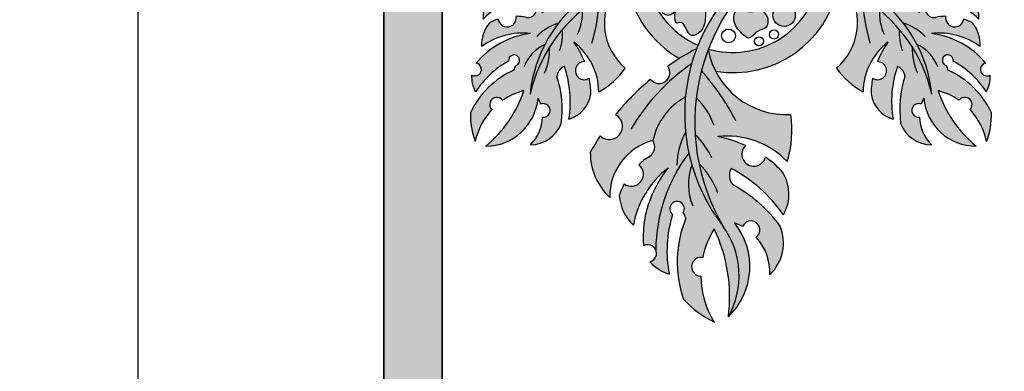
# Model space of a CAD drawing. Units: inches. Extents: x 3008 to 4088, y 1255 to 2137.
# Tile 12 of 30: x 3008 to 3093, y 1844 to 1874. Entities that reach past the tile are written whole.
import ezdxf

# ---------------------------------------------------------------- set-up
doc = ezdxf.new("R2010")
doc.units = ezdxf.units.IN
for name, color, linetype, lineweight in [('A-ANNO-DIMS', 2, 'Continuous', 18), ('C-PROP', 1, 'Continuous', 35), ('C-PROP-PATT', 9, 'Continuous', 13), ('estofado', 7, 'Continuous', 25), ('L-PLNT', 3, 'Continuous', 13)]:
    doc.layers.add(name, color=color, linetype=linetype, lineweight=lineweight)
doc.styles.get("Standard").update_dxf_attribs({"font": 'arial.ttf'})
doc.dimstyles.new('ISO-25', dxfattribs={"dimtxt": 8, "dimasz": 2.5, "dimexe": 1.25, "dimexo": 0.625, "dimtad": 1, "dimdec": 1, "dimlunit": 3, "dimtxsty": 'Standard', "dimcen": 2.5, "dimadec": 0, "dimazin": 0, "dimtfac": 1, "dimtdec": 1, "dimtmove": 0, "dimatfit": 3, "dimfxl": 1, "dimarcsym": 0})

# ---------------------------------------------------------------- blocks, each defined once
blk = doc.blocks.new('*D2')
at = {"layer": 'A-ANNO-DIMS', "color": 0, "lineweight": -2, "transparency": 16777216}
for p, q in [((3039.041, 2003.966), (3017.26, 2003.966)), ((3018.51, 2001.466), (3018.51, 1346.466)), ((3039.041, 1343.966), (3017.26, 1343.966))]:
    blk.add_line(p, q, dxfattribs=at)
at = {"layer": 'A-ANNO-DIMS', "color": 0, "transparency": 16777216}
for points in [[(3018.093, 2001.466), (3018.927, 2001.466), (3018.51, 2003.966)], [(3018.093, 1346.466), (3018.927, 1346.466), (3018.51, 1343.966)]]:
    blk.add_solid(points, dxfattribs=at)
at = {"layer": 'Defpoints', "color": 0, "transparency": 16777216}
for p in [(3039.666, 2003.966), (3018.51, 1343.966), (3039.666, 1343.966)]:
    blk.add_point(p, dxfattribs=at)
at = {"layer": 'A-ANNO-DIMS', "color": 0, "transparency": 16777216, "insert": (3013.817, 1673.966), "char_height": 8, "attachment_point": 5, "rotation": 90}
blk.add_mtext("55'", dxfattribs=at)
blk = doc.blocks.new('Novo Cashepo')
at = {"layer": 'estofado', "ltscale": 0.1}
h = blk.add_hatch(color=256, dxfattribs=at)
h.set_gradient(color1=(108, 164, 86), color2=(79, 120, 63), one_color=1, tint=0.36, name='CYLINDER')
h.paths.add_polyline_path([(0.2827, 0.4266, -0.314907), (0.2643, 0.3891, -0.122145), (0.2167, 0.5593, 0.291545), (0.1604, 0.4626, 0.043027), (0.1756, 0.4118, -1.339402), (0.202, 0.3602, 0.060072), (0.2488, 0.3031, -0.231117), (0.1355, 0.4506, 0.11449), (0.0635, 0.3561, -0.376746), (0.1502, 0.1049, 0.228124), (0.3602, 0.5016, -0.2613), (0.1736, 0.0872, 0.033062), (0.2588, 0.0848, -0.981895), (0.3134, 0.0893, 0.048855), (0.4361, 0.1168, -1.138233), (0.4978, 0.1407, 0.018864), (0.5414, 0.1623, 0.208979), (0.5618, 0.2847, -0.346636), (0.3922, 0.2224, -0.42625), (0.4225, 0.2519, 0.04537), (0.4552, 0.2547, -0.994855), (0.5125, 0.2753, 0.044381), (0.539, 0.2936, 0.18118), (0.5496, 0.3761, -0.18833), (0.3972, 0.3019, 0.191426), (0.5567, 0.4338, -1.174476), (0.5643, 0.4761, 0.140528), (0.5404, 0.529, -0.125367), (0.4517, 0.4068, -2.245001), (0.4262, 0.4175, -0.031976), (0.4282, 0.4328, 0.181425), (0.5443, 0.6013, 0.094503), (0.51, 0.6925, -0.138196), (0.476, 0.5769, -1.074478), (0.4463, 0.5393, -0.088291), (0.3828, 0.4942, -0.144087), (0.473, 0.7006, 0.388768), (0.3315, 0.5094, -0.041945), (0.3192, 0.5282, -1.340573), (0.3051, 0.5692, -0.196063), (0.327, 0.668, 0.307628), (0.2389, 0.5784, 0.111291)])
h = blk.add_hatch(color=256, dxfattribs=at)
h.set_gradient(color1=(108, 164, 86), color2=(102, 154, 81), one_color=1, tint=0.46, name='CYLINDER')
h.paths.add_polyline_path([(-0.0809, 0.1926, 0.033062), (-0.0785, 0.2778, -0.981895), (-0.0829, 0.3324, 0.048855), (-0.1105, 0.4551, -1.138233), (-0.1344, 0.5168, 0.018864), (-0.1559, 0.5604, 0.208979), (-0.2783, 0.5808, -0.346636), (-0.2161, 0.4112, -0.42625), (-0.2455, 0.4415, 0.04537), (-0.2484, 0.4742, -0.994855), (-0.269, 0.5315, 0.044381), (-0.2872, 0.5579, 0.18118), (-0.3697, 0.5686, -0.18833), (-0.2956, 0.4161, 0.191426), (-0.4275, 0.5757, -1.174476), (-0.4698, 0.5832, 0.140528), (-0.5227, 0.5593, -0.125367), (-0.4005, 0.4706, -2.245001), (-0.4112, 0.4452, -0.031976), (-0.4264, 0.4471, 0.181425), (-0.595, 0.5633, 0.094503), (-0.6862, 0.529, -0.138196), (-0.5706, 0.495, -1.074478), (-0.5329, 0.4652, -0.088291), (-0.4878, 0.4018, -0.144087), (-0.6943, 0.4919, 0.388768), (-0.503, 0.3504, -0.041945), (-0.5218, 0.3381, -1.340573), (-0.5628, 0.324, -0.196063), (-0.6617, 0.346, 0.307628), (-0.5721, 0.2579, 0.111291), (-0.4203, 0.3017, -0.314907), (-0.3828, 0.2833, -0.122145), (-0.553, 0.2356, 0.291545), (-0.4562, 0.1793, 0.043027), (-0.4055, 0.1946, -1.339402), (-0.3539, 0.2209, 0.060072), (-0.2968, 0.2677, -0.231117), (-0.4442, 0.1544, 0.11449), (-0.3498, 0.0824, -0.376746), (-0.0985, 0.1691, 0.228124), (-0.4952, 0.3792, -0.2613)])
h = blk.add_hatch(color=256, dxfattribs=at)
h.set_gradient(color1=(166, 115, 84), color2=(109, 75, 55), one_color=1, tint=0.32, name='INVCYLINDER')
h.paths.add_polyline_path([(0.3602, 0.5016, -0.309503), (0.0116, 0.0322, 0.812635), (0.0173, 0.012, 0.364481)])
h = blk.add_hatch(color=256, dxfattribs=at)
h.set_gradient(color1=(166, 115, 84), color2=(109, 75, 55), one_color=1, tint=0.32, name='INVCYLINDER')
h.paths.add_polyline_path([(-0.0186, 0.0079, 0.872708), (-0.0001, 0.0132, 0.378997), (-0.4952, 0.3792, -0.322151)])
h = blk.add_hatch(color=256, dxfattribs=at)
h.set_gradient(color1=(185, 193, 193), color2=(81, 92, 92), one_color=1, tint=0.34, name='CURVED')
h.paths.add_polyline_path([(0.1525, 0.1108, 0.06904), (0.1645, 0.1649, 0.288006), (-0.0787, 0.2226, -0.011646), (-0.0809, 0.1926, -0.009266), (-0.0709, 0.1786, -0.341204)])
h = blk.add_hatch(color=256, dxfattribs=at)
h.set_gradient(color1=(185, 193, 193), color2=(81, 92, 92), one_color=1, tint=0.34, name='CURVED')
h.paths.add_polyline_path([(-0.0966, 0.1665, 0.00155), (-0.0985, 0.1691, 0.067559), (-0.151, 0.1827, 0.253608), (-0.2368, -0.0242, -0.036817), (-0.1935, -0.0138, -0.290631)])
h = blk.add_hatch(color=256, dxfattribs=at)
h.set_gradient(color1=(179, 165, 128), color2=(150, 134, 90), one_color=1, tint=0.47)
h.paths.add_polyline_path([(-0.0466, 0.1604, -1), (0.0024, 0.1604, -1)])
h = blk.add_hatch(color=256, dxfattribs=at)
h.set_gradient(color1=(179, 165, 128), color2=(150, 134, 90), one_color=1, tint=0.47)
h.paths.add_polyline_path([(-0.113, 0.1431, 1), (-0.0932, 0.1431, 1)])
h = blk.add_hatch(color=256, dxfattribs=at)
h.set_gradient(color1=(179, 165, 128), color2=(150, 134, 90), one_color=1, tint=0.47)
h.paths.add_polyline_path([(0.0333, 0.1194, 1), (0.0824, 0.1194, 1)])
h = blk.add_hatch(color=256, dxfattribs=at)
h.set_gradient(color1=(179, 165, 128), color2=(150, 134, 90), one_color=1, tint=0.47)
h.paths.add_polyline_path([(-0.149, 0.1152, 1), (-0.1291, 0.1152, 1)])
h = blk.add_hatch(color=256, dxfattribs=at)
h.set_gradient(color1=(179, 165, 128), color2=(150, 134, 90), one_color=1, tint=0.47)
edge = h.paths.add_edge_path()
edge.add_spline(control_points=[(-0.126, 0.0391), (-0.128, 0.0314), (-0.132, 0.0156), (-0.099, 0.0101), (-0.0817, 0.025), (-0.0594, 0.0483), (-0.0851, 0.062), (-0.0856, 0.0869), (-0.1113, 0.0892), (-0.1235, 0.079), (-0.1379, 0.0613), (-0.1214, 0.0568), (-0.124, 0.0467), (-0.126, 0.0391)], knot_values=[0, 0, 0, 0, 0.020201, 0.040881, 0.075874, 0.093984, 0.117931, 0.138882, 0.158108, 0.177537, 0.194687, 0.200618, 0.219249, 0.219249, 0.219249, 0.219249], degree=3, periodic=0)
h = blk.add_hatch(color=256, dxfattribs=at)
h.set_gradient(color1=(185, 193, 193), color2=(81, 92, 92), one_color=1, tint=0.34, name='CURVED')
h.paths.add_polyline_path([(0.1736, 0.0872, -0.003321), (0.1687, 0.0836, -0.134103), (0.1873, -0.0153, -0.036923), (0.2304, -0.0269, 0.121396), (0.2162, 0.0846, -0.016535)])
h = blk.add_hatch(color=256, dxfattribs=at)
h.set_gradient(color1=(179, 165, 128), color2=(150, 134, 90), one_color=1, tint=0.47)
h.paths.add_polyline_path([(0.0244, 0.0622, 1), (-0.0057, 0.0622, 1)])
h = blk.add_hatch(color=256, dxfattribs=at)
h.set_gradient(color1=(179, 165, 128), color2=(150, 134, 90), one_color=1, tint=0.47)
h.paths.add_polyline_path([(0.1562, 0.0298, 1), (0.1262, 0.0298, 1)])
h = blk.add_hatch(color=256, dxfattribs=at)
h.set_gradient(color1=(166, 115, 84), color2=(109, 75, 55), one_color=1, tint=0.32, name='INVCYLINDER')
h.paths.add_polyline_path([(0.0994, 0.0192, 0.726279), (0.0923, 0.0227, 0.000011), (0.0923, 0.0227, 0.454782), (-0.024, -0.5707, -0.387777)])
h = blk.add_hatch(color=256, dxfattribs=at)
h.set_gradient(color1=(179, 165, 128), color2=(150, 134, 90), one_color=1, tint=0.47)
h.paths.add_polyline_path([(-0.0448, 0.022, 1), (-0.0748, 0.022, 1)])
h = blk.add_hatch(color=256, dxfattribs=at)
h.set_gradient(color1=(179, 165, 128), color2=(150, 134, 90), one_color=1, tint=0.47)
h.paths.add_polyline_path([(0.1828, 0.0084, 1), (0.1527, 0.0084, 1)])
h = blk.add_hatch(color=256, dxfattribs=at)
h.set_gradient(color1=(179, 165, 128), color2=(150, 134, 90), one_color=1, tint=0.47)
h.paths.add_polyline_path([(-0.1713, 0.0047, 1), (-0.1912, 0.0047, 1)])
h = blk.add_hatch(color=256, dxfattribs=at)
h.set_gradient(color1=(179, 165, 128), color2=(150, 134, 90), one_color=1, tint=0.47)
h.paths.add_polyline_path([(-0.0766, 0.0036, 1), (-0.0965, 0.0036, 1)])
h = blk.add_hatch(color=256, dxfattribs=at)
h.set_gradient(color1=(179, 165, 128), color2=(150, 134, 90), one_color=1, tint=0.47)
h.paths.add_polyline_path([(0.0176, -0.0063, 1), (-0.0023, -0.0063, 1)])
h = blk.add_hatch(color=256, dxfattribs=at)
h.set_gradient(color1=(166, 115, 84), color2=(109, 75, 55), one_color=1, tint=0.32, name='INVCYLINDER')
h.paths.add_polyline_path([(-0.0708, -0.0241, 0.529291), (-0.0712, -0.0189, 0.456534), (-0.4459, -0.2817, -0.387777)])
h = blk.add_hatch(color=256, dxfattribs=at)
h.set_gradient(color1=(179, 165, 128), color2=(150, 134, 90), one_color=1, tint=0.47)
h.paths.add_polyline_path([(-0.0152, -0.0149, 1), (-0.0351, -0.0149, 1)])
h = blk.add_hatch(color=256, dxfattribs=at)
h.set_gradient(color1=(166, 115, 84), color2=(109, 75, 55), one_color=1, tint=0.32, name='INVCYLINDER')
h.paths.add_polyline_path([(0.4314, -0.2817, 0.456534), (0.0566, -0.0189, 0.529291), (0.0563, -0.0241, -0.387777)])
h = blk.add_hatch(color=256, dxfattribs=at)
h.set_gradient(color1=(108, 164, 86), color2=(62, 94, 49), one_color=1, tint=0.28, name='CURVED')
h.paths.add_polyline_path([(-0.5633, -0.214, -1.174476), (-0.5734, -0.2402, 0.140528), (-0.5646, -0.277, -0.125367), (-0.4927, -0.2097, -2.245001), (-0.4777, -0.2197, -0.031976), (-0.4809, -0.2292, 0.181425), (-0.5761, -0.3228, 0.094503), (-0.5654, -0.3855, -0.138196), (-0.5293, -0.3156, -1.074478), (-0.5056, -0.2952, -0.088291), (-0.4594, -0.2742, -0.144087), (-0.5427, -0.3952, 0.388768), (-0.4284, -0.2902, -0.041945), (-0.4229, -0.3038, -1.340573), (-0.4189, -0.3318, -0.196063), (-0.4452, -0.3924, 0.307628), (-0.3777, -0.3459, 0.111291), (-0.387, -0.2433, -0.314907), (-0.3706, -0.2216, -0.122145), (-0.3611, -0.3364, 0.291545), (-0.3131, -0.2814, 0.043027), (-0.3166, -0.247, -1.339402), (-0.3271, -0.2108, 0.060072), (-0.35, -0.1684, -0.231117), (-0.2957, -0.2768, 0.11449), (-0.2379, -0.2252, -0.376746), (-0.2623, -0.0537, 0.228124), (-0.4459, -0.2817, -0.2613), (-0.2752, -0.0394, 0.033062), (-0.3295, -0.0274, -0.981895), (-0.365, -0.0235, 0.048855), (-0.4469, -0.026, -1.138233), (-0.4894, -0.0336, 0.018864), (-0.52, -0.042, 0.208979), (-0.5481, -0.1179, -0.346636), (-0.4319, -0.099, -0.42625), (-0.4549, -0.1141, 0.04537), (-0.4762, -0.1119, -0.994855), (-0.5154, -0.118, 0.044381), (-0.5346, -0.1264, 0.18118), (-0.5516, -0.1779, -0.18833), (-0.4449, -0.1493, 0.191426)])
h = blk.add_hatch(color=256, dxfattribs=at)
h.set_gradient(color1=(185, 193, 193), color2=(81, 92, 92), one_color=1, tint=0.34, name='CURVED')
h.paths.add_polyline_path([(-0.1917, -0.0292, 0.03292), (-0.2343, -0.0418, 0.221446), (-0.1198, -0.2039, -0.019377), (-0.0822, -0.1825, -0.005069), (-0.0793, -0.175, -0.256969)])
h = blk.add_hatch(color=256, dxfattribs=at)
h.set_gradient(color1=(179, 165, 128), color2=(150, 134, 90), one_color=1, tint=0.47)
h.paths.add_polyline_path([(-0.1275, -0.0533, 1), (-0.1765, -0.0533, 1)])
h = blk.add_hatch(color=256, dxfattribs=at)
h.set_gradient(color1=(179, 165, 128), color2=(150, 134, 90), one_color=1, tint=0.47)
h.paths.add_polyline_path([(-0.0439, -0.0322, 1), (-0.0638, -0.0322, 1)])
h = blk.add_hatch(color=256, dxfattribs=at)
h.set_gradient(color1=(185, 193, 193), color2=(81, 92, 92), one_color=1, tint=0.34, name='CURVED')
h.paths.add_polyline_path([(0.1853, -0.0311, -0.449638), (-0.0565, -0.1832, 0.000699), (-0.0569, -0.1844, 0.072477), (-0.0408, -0.2319, 0.40511), (0.2276, -0.0448, 0.032975)])
h = blk.add_hatch(color=256, dxfattribs=at)
h.set_gradient(color1=(179, 165, 128), color2=(150, 134, 90), one_color=1, tint=0.47)
h.paths.add_polyline_path([(-0.0194, -0.0559, 1), (-0.0495, -0.0559, 1)])
h = blk.add_hatch(color=256, dxfattribs=at)
h.set_gradient(color1=(179, 165, 128), color2=(150, 134, 90), one_color=1, tint=0.47)
h.paths.add_polyline_path([(0.0597, -0.0435, 1), (0.0398, -0.0435, 1)])
h = blk.add_hatch(color=256, dxfattribs=at)
h.set_gradient(color1=(179, 165, 128), color2=(150, 134, 90), one_color=1, tint=0.47)
h.paths.add_polyline_path([(0.0939, -0.0406, 1), (0.0639, -0.0406, 1)])
h = blk.add_hatch(color=256, dxfattribs=at)
h.set_gradient(color1=(179, 165, 128), color2=(150, 134, 90), one_color=1, tint=0.47)
h.paths.add_polyline_path([(0.1743, -0.0543, 1), (0.1253, -0.0543, 1)])
h = blk.add_hatch(color=256, dxfattribs=at)
h.set_gradient(color1=(108, 164, 86), color2=(154, 193, 138), one_color=1, tint=0.65, name='HEMISPHERICAL')
h.paths.add_polyline_path([(0.4174, -0.099, -0.346636), (0.5336, -0.1179, 0.208979), (0.5055, -0.042, 0.018864), (0.4749, -0.0336, -1.138233), (0.4324, -0.026, 0.048855), (0.3504, -0.0235, -0.981895), (0.3149, -0.0274, 0.033062), (0.2607, -0.0394, -0.2613), (0.4314, -0.2817, 0.228124), (0.2478, -0.0537, -0.376746), (0.2234, -0.2252, 0.11449), (0.2812, -0.2768, -0.231117), (0.3355, -0.1684, 0.060072), (0.3126, -0.2108, -1.339402), (0.3021, -0.247, 0.043027), (0.2986, -0.2814, 0.291545), (0.3466, -0.3364, -0.122145), (0.3561, -0.2216, -0.314907), (0.3725, -0.2433, 0.111291), (0.3632, -0.3459, 0.307628), (0.4307, -0.3924, -0.196063), (0.4044, -0.3318, -1.340573), (0.4084, -0.3038, -0.041945), (0.4139, -0.2902, 0.388768), (0.5282, -0.3952, -0.144087), (0.4449, -0.2742, -0.088291), (0.4911, -0.2952, -1.074478), (0.5148, -0.3156, -0.138196), (0.5509, -0.3855, 0.094503), (0.5616, -0.3228, 0.181425), (0.4664, -0.2292, -0.031976), (0.4632, -0.2197, -2.245001), (0.4782, -0.2097, -0.125367), (0.5501, -0.277, 0.140528), (0.5589, -0.2402, -1.174476), (0.5488, -0.214, 0.191426), (0.4304, -0.1493, -0.18833), (0.5371, -0.1779, 0.18118), (0.5201, -0.1264, 0.044381), (0.5009, -0.118, -0.994855), (0.4617, -0.1119, 0.04537), (0.4404, -0.1141, -0.42625)])
h = blk.add_hatch(color=256, dxfattribs=at)
h.set_gradient(color1=(179, 165, 128), color2=(150, 134, 90), one_color=1, tint=0.47)
h.paths.add_polyline_path([(-0.1294, -0.0948, 1), (-0.1594, -0.0948, 1)])
h = blk.add_hatch(color=256, dxfattribs=at)
h.set_gradient(color1=(179, 165, 128), color2=(150, 134, 90), one_color=1, tint=0.47)
edge = h.paths.add_edge_path()
edge.add_spline(control_points=[(-0.1055, -0.1384), (-0.1019, -0.1456), (-0.0945, -0.16), (-0.0661, -0.1423), (-0.063, -0.1197), (-0.0617, -0.0875), (-0.09, -0.0942), (-0.1068, -0.0758), (-0.1276, -0.0911), (-0.13, -0.1069), (-0.1291, -0.1297), (-0.1137, -0.1221), (-0.1091, -0.1314), (-0.1055, -0.1384)], knot_values=[0, 0, 0, 0, 0.020201, 0.040881, 0.075874, 0.093984, 0.117931, 0.138882, 0.158108, 0.177537, 0.194687, 0.200618, 0.219249, 0.219249, 0.219249, 0.219249], degree=3, periodic=0)
h = blk.add_hatch(color=256, dxfattribs=at)
h.set_gradient(color1=(179, 165, 128), color2=(150, 134, 90), one_color=1, tint=0.47)
h.paths.add_polyline_path([(0.1333, -0.1092, 1), (0.0843, -0.1092, 1)])
h = blk.add_hatch(color=256, dxfattribs=at)
h.set_gradient(color1=(179, 165, 128), color2=(150, 134, 90), one_color=1, tint=0.47)
edge = h.paths.add_edge_path()
edge.add_spline(control_points=[(0.0251, -0.0997), (0.0173, -0.0977), (0.0016, -0.0937), (-0.004, -0.1268), (0.011, -0.1441), (0.0343, -0.1664), (0.0479, -0.1407), (0.0728, -0.1402), (0.0751, -0.1145), (0.0649, -0.1023), (0.0473, -0.0879), (0.0427, -0.1044), (0.0327, -0.1017), (0.0251, -0.0997)], knot_values=[0, 0, 0, 0, 0.020201, 0.040881, 0.075874, 0.093984, 0.117931, 0.138882, 0.158108, 0.177537, 0.194687, 0.200618, 0.219249, 0.219249, 0.219249, 0.219249], degree=3, periodic=0)
h = blk.add_hatch(color=256, dxfattribs=at)
h.set_gradient(color1=(108, 164, 86), color2=(128, 178, 108), one_color=1, tint=0.56, name='CYLINDER')
h.paths.add_polyline_path([(-0.0931, -0.2153, -0.021499), (-0.0822, -0.1825, 0.033062), (-0.1452, -0.2207, -0.981895), (-0.1828, -0.2494, 0.048855), (-0.259, -0.3268, -1.138233), (-0.2927, -0.373, 0.018864), (-0.3143, -0.409, 0.208979), (-0.2718, -0.5074, -0.346636), (-0.1778, -0.383, -0.218356), (-0.1066, -0.288, -0.045186), (-0.0935, -0.2168, -0.00127), (-0.0946, -0.2163, -0.001036)])
h = blk.add_hatch(color=256, dxfattribs=at)
h.set_gradient(color1=(108, 164, 86), color2=(128, 178, 108), one_color=1, tint=0.56, name='CYLINDER')
h.paths.add_polyline_path([(0.1153, -0.4286, 0.11449), (0.1235, -0.3263, -0.376746), (-0.0569, -0.1844, 0.228124), (-0.024, -0.5707, -0.289779), (-0.0128, -0.768, 0.388768), (0.0005, -0.5629, -0.041945), (0.0182, -0.5708, -1.340573), (0.0477, -0.594, -0.196063), (0.0779, -0.676, 0.307628), (0.1, -0.5698, 0.111291), (-0.0028, -0.48, -0.314907), (-0.0069, -0.4442, -0.122145), (0.1072, -0.5455, 0.291545), (0.1029, -0.4489, 0.043027), (0.0681, -0.4192, -1.339402), (0.0248, -0.3941, 0.060072), (-0.0358, -0.3745, -0.231117)])
h = blk.add_hatch(color=256, dxfattribs=at)
h.set_gradient(color1=(108, 164, 86), color2=(128, 178, 108), one_color=1, tint=0.56, name='CYLINDER')
h.paths.add_polyline_path([(-0.186, -0.4185, 0.04537), (-0.2084, -0.4358, -0.994855), (-0.2404, -0.4776, 0.044381), (-0.2511, -0.5032, 0.18118), (-0.2202, -0.5681, -0.18833), (-0.1442, -0.443, 0.191426), (-0.1984, -0.6134, -0.461932), (-0.1711, -0.6221, -0.164855), (-0.099, -0.4106, -0.076989), (-0.1066, -0.288, 0.218356), (-0.1778, -0.383, -0.42625)])
h = blk.add_hatch(color=256, dxfattribs=at)
h.set_gradient(color1=(108, 164, 86), color2=(128, 178, 108), one_color=1, tint=0.56, name='CYLINDER')
h.paths.add_polyline_path([(-0.1111, -0.7292, 0.094503), (-0.0435, -0.7794, -0.138196), (-0.0729, -0.6796, -1.074478), (-0.0689, -0.6383, -0.088291), (-0.0439, -0.5759, -0.144087), (-0.0128, -0.768, 0.289779), (-0.024, -0.5707, -0.111568), (-0.099, -0.4106, 0.164855), (-0.1711, -0.6221, -0.461932), (-0.1841, -0.6476, 0.140528), (-0.142, -0.6749, -0.125367), (-0.1347, -0.5446, -2.245001), (-0.1112, -0.5405, -0.031976), (-0.1055, -0.5525, 0.181425)])
for centre, radius in [((-0.0221, 0.1604), 0.0245), ((0.0395, 0.1667), 0.015), ((-0.1031, 0.1431), 0.00994), ((0.0215, 0.1368), 0.015), ((0.0578, 0.1194), 0.0245), ((0.1044, 0.1338), 0.015), ((-0.1391, 0.1152), 0.00994), ((-0.1006, 0.1127), 0.015), ((-0.0753, 0.0931), 0.015), ((-0.0182, 0.1092), 0.00994), ((0.0145, 0.1013), 0.015), ((0.0993, 0.0941), 0.015), ((-0.1296, 0.0906), 0.00994), ((-0.0066, 0.0836), 0.00994), ((0.0432, 0.0739), 0.015), ((0.0724, 0.0784), 0.00994), ((-0.1435, 0.0709), 0.00994), ((-0.0657, 0.0663), 0.00994), ((0.0093, 0.0622), 0.015), ((-0.155, 0.0346), 0.0245), ((0.1412, 0.0298), 0.015), ((0.1627, 0.0543), 0.00994), ((-0.0598, 0.022), 0.015), ((0.1127, 0.0289), 0.00994), ((0.1678, 0.0084), 0.015), ((-0.1813, 0.0047), 0.00994), ((-0.1282, 0.0051), 0.00994), ((-0.0866, 0.0036), 0.00994), ((-0.0635, -0.0053), 0.00994), ((-0.0398, 0.002), 0.00994), ((0.0077, -0.0063), 0.00994), ((0.0352, 0.0026), 0.00994), ((0.0994, 0.0024), 0.00994), ((0.127, 0.0055), 0.00994), ((-0.0252, -0.0149), 0.00994), ((-0.0085, -0.0314), 0.00994), ((-0.152, -0.0533), 0.0245), ((-0.1111, -0.0406), 0.015), ((-0.0806, -0.0403), 0.00994), ((-0.0539, -0.0322), 0.00994), ((-0.0345, -0.0559), 0.015), ((0.0498, -0.0435), 0.00994), ((0.0789, -0.0406), 0.015), ((0.1498, -0.0543), 0.0245), ((-0.0774, -0.0694), 0.00994), ((0.0329, -0.0722), 0.015), ((0.0754, -0.0779), 0.015), ((0.1084, -0.0629), 0.015), ((-0.1444, -0.0948), 0.015), ((0.1088, -0.1092), 0.0245), ((-0.0125, -0.1547), 0.015), ((0.0867, -0.1514), 0.00994), ((0.0538, -0.1663), 0.00994)]:
    blk.add_circle(centre, radius, dxfattribs=at)
for centre, radius, start, end in [((0.5066, 0.5278), 0.1761, 101.0186, 185.9966), ((0.7787, 0.4442), 0.399, 140.0122, 172.8088), ((0.2879, 0.6951), 0.2222, 327.8752, 359.3481), ((0.2881, 0.557), 0.26, 9.8207, 31.4151), ((0.3489, 0.5584), 0.1118, 101.2825, 169.6799), ((0.4372, 0.5917), 0.134, 145.305, 189.6765), ((-0.4545, 0.479), 0.1053, 98.3059, 130.3029), ((-0.4492, 0.576), 0.0218, 160.6631, 359.0131), ((-0.2404, 0.4305), 0.1549, 56.9429, 104.1578), ((-0.3548, 0.4565), 0.1459, 341.9118, 58.3844), ((0.2616, 0.6719), 0.2914, 304.8613, 345.9935), ((-0.5506, 0.307), 0.26, 99.8207, 121.4151), ((-0.6655, 0.2806), 0.2914, 34.8613, 75.9935), ((-0.6357, 0.2751), 0.3059, 39.7257, 68.3087), ((-0.5622, 0.33), 0.2802, 17.9062, 61.2534), ((-0.3427, 0.4531), 0.1185, 62.1153, 103.1932), ((-0.5278, 0.3974), 0.233, 4.6076, 47.2701), ((-0.7231, 0.2531), 0.6451, 24.1234, 28.4463), ((0.2645, 0.4667), 0.1042, 117.2921, 182.3073), ((0.5836, 0.5703), 0.3671, 181.7055, 209.5612), ((0.5976, 0.5997), 0.3593, 183.393, 208.7944), ((0.306, 0.5466), 0.0226, 92.4292, 305.5449), ((0.4625, 0.557), 0.024, 227.5673, 55.7919), ((-0.4269, 0.4422), 0.1813, 29.481, 39.6456), ((0.2879, 0.6951), 0.2222, 295.3016, 315.484), ((-0.6887, 0.3068), 0.2222, 57.8752, 89.3481), ((-0.2585, 0.5029), 0.0304, 110.1108, 289.5198), ((-0.1264, 0.4844), 0.0334, 103.7865, 298.5822), ((0.4372, 0.5917), 0.134, 208.2976, 217.9049), ((0.2562, 0.6421), 0.3059, 309.7257, 338.3087), ((0.4601, 0.4609), 0.1053, 8.3059, 40.3029), ((-0.5507, 0.4815), 0.024, 317.5673, 145.7919), ((-0.1569, 0.5215), 0.5175, 289.0066, 357.7964), ((-0.1024, 0.4607), 0.4645, 284.942, 5.0453), ((-0.4379, 0.7976), 0.399, 230.0122, 262.8088), ((-0.5214, 0.5256), 0.1761, 191.0186, 275.9966), ((-0.4269, 0.4422), 0.1813, 359.2754, 10.1496), ((0.5571, 0.4556), 0.0218, 70.6631, 269.0131), ((-0.6887, 0.3068), 0.2222, 25.3016, 45.484), ((-0.3944, 0.4531), 0.0186, 205.201, 109.1617), ((-0.7231, 0.2531), 0.6451, 7.0576, 18.2453), ((0.4622, 0.5257), 0.3083, 191.8137, 201.6687), ((-0.4035, 0.5652), 0.1203, 259.0186, 266.3445), ((-0.2163, 0.4404), 0.0293, 181.0153, 270.3634), ((-0.6263, 0.2061), 0.5206, 1.9256, 26.9542), ((0.303, 0.2481), 0.2627, 129.608, 155.7334), ((0.3431, 0.4928), 0.2118, 191.5061, 243.5602), ((0.311, 0.5686), 0.2802, 287.9062, 331.2534), ((0.5463, 0.4099), 0.1203, 169.0186, 176.3445), ((-0.4326, 0.2811), 0.1367, 36.1411, 80.3873), ((0.1964, 0.3899), 0.0302, 280.5489, 133.5686), ((0.2467, 0.421), 0.0364, 298.8789, 8.7972), ((0.5076, 0.3784), 0.1869, 165.9423, 193.4167), ((0.2622, 0.4389), 0.1367, 306.1411, 350.3873), ((0.4341, 0.4007), 0.0186, 115.201, 19.1617), ((-0.4031, 0.2432), 0.1817, 28.6905, 56.0246), ((-0.3847, 0.2462), 0.2195, 9.4944, 41.5537), ((-0.4544, -0.0835), 0.4645, 12.0191, 95.0453), ((-0.5151, -0.138), 0.5175, 16.3708, 87.7964), ((0.3785, 0.5342), 0.233, 274.6076, 317.2701), ((0.4342, 0.349), 0.1185, 332.1153, 13.1932), ((-0.5854, 0.4562), 0.134, 235.305, 279.6765), ((-0.5521, 0.3678), 0.1118, 191.2825, 259.6799), ((-0.5854, 0.4562), 0.134, 298.2976, 307.9049), ((-0.372, 0.5266), 0.1869, 255.9423, 283.4167), ((-0.0362, 0.1811), 0.2014, 337.7465, 60.3213), ((0.4622, 0.5257), 0.3083, 212.4488, 226.1997), ((-0.5402, 0.325), 0.0226, 182.4292, 35.5449), ((-0.0802, 0.3051), 0.0274, 95.6708, 273.5772), ((0.4824, 0.3139), 0.1936, 172.3137, 193.7119), ((-0.5933, 0.6166), 0.3593, 273.393, 298.7944), ((-0.4147, 0.2657), 0.0364, 28.8789, 98.7972), ((-0.3076, 0.5014), 0.1936, 262.3137, 283.7119), ((0.2242, 0.4094), 0.1817, 298.6905, 326.0246), ((-0.5639, 0.6026), 0.3671, 271.7055, 299.5612), ((0.8078, 0.234), 0.6217, 174.4084, 188.6615), ((0.4375, 0.3611), 0.1459, 251.9118, 328.3844), ((0.4839, 0.2649), 0.0304, 20.1108, 199.5198), ((0.4233, 0.4332), 0.1813, 299.481, 309.6456), ((0.4116, 0.2468), 0.1549, 326.9429, 14.1578), ((-0.4865, 0.362), 0.2118, 281.5061, 333.5602), ((-0.5193, 0.4811), 0.3083, 302.4488, 316.1997), ((-0.2254, 0.4264), 0.1711, 255.544, 283.8081), ((-0.7231, 0.2531), 0.6451, 354.6159, 2.1904), ((0.4075, 0.2318), 0.1711, 165.544, 193.8081), ((-0.3836, 0.2154), 0.0302, 10.5489, 223.5686), ((0.4215, 0.2226), 0.0293, 91.0153, 180.3634), ((0.4233, 0.4332), 0.1813, 269.2754, 280.1496), ((-0.4604, 0.2834), 0.1042, 207.2921, 272.3073), ((-0.003, 0.0001), 0.235, 44.5248, 108.7916), ((0.2272, 0.3911), 0.2195, 279.4944, 311.5537), ((-0.5193, 0.4811), 0.3083, 281.8137, 291.6687), ((-0.2276, 0.8267), 0.6217, 264.4084, 278.6615), ((-0.1748, -0.0173), 0.2014, 67.7465, 150.3213), ((-0.003, 0.0001), 0.235, 129.0122, 185.9347), ((-0.003, 0.0001), 0.1909, 35.4554, 110.8148), ((-0.2418, 0.3219), 0.2627, 219.608, 245.7334), ((-0.003, 0.0001), 0.1909, 119.3518, 184.1737), ((0.1872, 0.6326), 0.5206, 271.9256, 296.9542), ((0.4654, 0.1328), 0.0334, 13.7865, 208.5822), ((0.2342, 0.7294), 0.6451, 294.1234, 298.4463), ((0.2862, 0.0866), 0.0274, 5.6708, 183.5772), ((0.2342, 0.7294), 0.6451, 277.0576, 288.2453), ((0.2342, 0.7294), 0.6451, 264.6159, 272.1904), ((-0.003, 0.0001), 0.1909, 355.3819, 25.9338), ((-0.003, 0.0001), 0.235, 353.3979, 21.0844), ((0.2929, -0.3247), 0.4012, 120.0005, 217.8213), ((0.0166, 0.0227), 0.0107, 117.5535, 273.9476), ((0.0953, 0.0198), 0.00417, 352.069, 136.0321), ((0.3609, -0.3433), 0.447, 125.7916, 210.5723), ((-0.0097, 0.0118), 0.00971, 203.8853, 8.3312), ((-0.1446, -0.3127), 0.3029, 76.2995, 174.1203), ((-0.1172, -0.3583), 0.3375, 82.0906, 166.8713), ((-0.0727, -0.0216), 0.00315, 308.368, 92.3311), ((0.0582, -0.0216), 0.00315, 87.6689, 231.632), ((0.1027, -0.3583), 0.3375, 13.1287, 97.9094), ((0.1301, -0.3127), 0.3029, 5.8797, 103.7005), ((-0.4473, -0.1122), 0.101, 136.0179, 183.2328), ((-0.3933, -0.4432), 0.4207, 103.1984, 107.5212), ((-0.4677, -0.0325), 0.0217, 182.8615, 17.6572), ((-0.3933, -0.4432), 0.4207, 86.1325, 97.3203), ((-0.3472, -0.0251), 0.0179, 174.7458, 352.6522), ((-0.3933, -0.4432), 0.4207, 73.6909, 81.2654), ((-0.003, 0.0001), 0.235, 190.2712, 240.2168), ((-0.003, 0.0001), 0.1909, 188.82, 246.4657), ((-0.003, 0.0001), 0.1909, 253.7485, 350.5904), ((0.3788, -0.4432), 0.4207, 98.7346, 106.3091), ((0.3327, -0.0251), 0.0179, 187.3478, 5.2542), ((0.3788, -0.4432), 0.4207, 82.6797, 93.8675), ((0.4531, -0.0325), 0.0217, 162.3428, 357.1385), ((0.3788, -0.4432), 0.4207, 72.4788, 76.8016), ((0.4328, -0.1122), 0.101, 356.7672, 43.9821), ((-0.3513, -0.387), 0.3395, 81.0006, 106.0292), ((-0.1524, -0.1255), 0.1313, 146.8215, 229.3963), ((-0.003, 0.0001), 0.235, 260.7676, 348.9809), ((0.1379, -0.1255), 0.1313, 310.6037, 33.1785), ((0.3368, -0.387), 0.3395, 73.9708, 98.9994), ((-0.3471, -0.2274), 0.1431, 88.5693, 120.6287), ((-0.6994, -0.055), 0.4054, 343.4834, 357.7365), ((0.6849, -0.055), 0.4054, 182.2635, 196.5166), ((0.3325, -0.2274), 0.1431, 59.3713, 91.4307), ((-0.478, -0.1822), 0.0952, 60.9868, 137.4594), ((-0.4506, -0.0955), 0.0191, 260.0903, 349.4383), ((-0.4428, -0.1031), 0.1116, 334.6189, 2.8831), ((0.4283, -0.1031), 0.1116, 177.1169, 205.3811), ((0.4635, -0.1822), 0.0952, 42.5406, 119.0132), ((0.4361, -0.0955), 0.0191, 190.5617, 279.9097), ((-0.4744, -0.1749), 0.0773, 141.1903, 182.2681), ((-0.4778, -0.2301), 0.1183, 108.5559, 118.7205), ((-0.4958, -0.1149), 0.0199, 189.1858, 8.5947), ((-0.4778, -0.2301), 0.1183, 78.3504, 89.2246), ((-0.3474, -0.2395), 0.1185, 107.7654, 135.0996), ((0.3329, -0.2395), 0.1185, 44.9004, 72.2346), ((0.4633, -0.2301), 0.1183, 90.7754, 101.6496), ((0.4813, -0.1149), 0.0199, 171.4053, 350.8142), ((0.4633, -0.2301), 0.1183, 61.2795, 71.4441), ((0.4599, -0.1749), 0.0773, 357.7319, 38.8097), ((-0.4227, -0.3307), 0.1827, 96.9812, 140.3284), ((-0.4616, -0.3003), 0.1519, 83.6826, 126.345), ((-0.5009, -0.1464), 0.1263, 341.3887, 2.7869), ((0.4864, -0.1464), 0.1263, 177.2131, 198.6113), ((0.4471, -0.3003), 0.1519, 53.655, 96.3174), ((0.4082, -0.3307), 0.1827, 39.6716, 83.0188), ((-0.5141, -0.2845), 0.2011, 21.5237, 35.2746), ((-0.4338, -0.2782), 0.1381, 0.581, 52.6352), ((0.4193, -0.2782), 0.1381, 127.3648, 179.419), ((0.4996, -0.2845), 0.2011, 144.7254, 158.4763), ((-0.3754, -0.2537), 0.0892, 115.216, 159.4623), ((-0.525, -0.1846), 0.1219, 335.0173, 2.4916), ((0.1741, -0.6772), 0.5572, 117.3918, 124.9664), ((0.1141, -0.1526), 0.1739, 190.5225, 273.0973), ((0.5105, -0.1846), 0.1219, 177.5084, 204.9827), ((0.3608, -0.2537), 0.0892, 20.5377, 64.784), ((-0.5662, -0.2279), 0.0142, 239.7381, 78.088), ((-0.3966, -0.3845), 0.1995, 118.8007, 147.3836), ((-0.4807, -0.208), 0.0121, 284.2759, 188.2367), ((-0.3272, -0.2305), 0.0197, 89.6239, 302.6435), ((0.3127, -0.2305), 0.0197, 237.3565, 90.3761), ((0.4662, -0.208), 0.0121, 351.7633, 255.7241), ((0.3821, -0.3845), 0.1995, 32.6164, 61.1993), ((0.5517, -0.2279), 0.0142, 101.912, 300.2619), ((-0.4038, -0.4029), 0.19, 113.9363, 155.0685), ((-0.5537, -0.2), 0.0785, 338.0936, 345.4195), ((-0.3633, -0.2442), 0.0238, 107.9539, 177.8722), ((-0.5974, -0.2981), 0.2394, 350.7805, 18.6362), ((-0.3779, -0.1265), 0.1713, 298.683, 324.8084), ((0.1629, -0.585), 0.4497, 124.7016, 149.7302), ((-0.1643, -0.2347), 0.0237, 218.4468, 36.3532), ((-0.003, 0.0001), 0.235, 247.0716, 247.3627), ((-0.4741, -0.5856), 0.5369, 27.1843, 41.4375), ((0.3634, -0.1265), 0.1713, 215.1916, 241.317), ((0.5829, -0.2981), 0.2394, 161.3638, 189.2195), ((0.3487, -0.2442), 0.0238, 2.1278, 72.0461), ((0.5392, -0.2), 0.0785, 194.5805, 201.9064), ((0.3893, -0.4029), 0.19, 24.9315, 66.0637), ((-0.5048, -0.2433), 0.0687, 177.3808, 209.3779), ((-0.61, -0.3152), 0.2343, 352.4679, 17.8694), ((-0.5141, -0.2845), 0.2011, 0.8887, 10.7437), ((0.1741, -0.6772), 0.5572, 129.8335, 141.0213), ((0.4996, -0.2845), 0.2011, 169.2563, 179.1113), ((0.5955, -0.3152), 0.2343, 162.1306, 187.5321), ((0.4903, -0.2433), 0.0687, 330.6221, 2.6192), ((-0.7067, -0.1933), 0.2602, 309.0872, 341.8838), ((-0.4235, -0.4145), 0.1449, 104.3766, 124.559), ((0.4089, -0.4145), 0.1449, 55.441, 75.6234), ((0.6922, -0.1933), 0.2602, 198.1162, 230.9128), ((-0.5429, -0.2804), 0.1149, 270.0936, 355.0715), ((-0.5182, -0.3046), 0.0157, 36.6423, 224.8669), ((-0.5063, -0.3299), 0.0874, 17.3725, 26.9799), ((-0.3803, -0.2712), 0.0679, 286.3671, 351.3823), ((-0.0386, -0.4131), 0.1424, 118.5185, 167.7887), ((-0.1845, -0.3969), 0.1478, 18.3199, 46.584), ((0.3657, -0.2712), 0.0679, 188.6177, 253.6329), ((0.4918, -0.3299), 0.0874, 153.0201, 162.6275), ((0.5283, -0.2804), 0.1149, 184.9285, 269.9064), ((0.5037, -0.3046), 0.0157, 315.1331, 143.3577), ((-0.4235, -0.4145), 0.1449, 136.9502, 168.4231), ((-0.4167, -0.3172), 0.0148, 261.5041, 114.6198), ((0.4022, -0.3172), 0.0148, 65.3802, 278.4959), ((0.4089, -0.4145), 0.1449, 11.5769, 43.0498), ((-0.4065, -0.3261), 0.1696, 178.8957, 200.49), ((-0.5063, -0.3299), 0.0874, 314.38, 358.7514), ((-0.2728, -0.352), 0.0288, 226.5625, 61.3582), ((-0.1009, -0.3599), 0.2269, 342.384, 8.5094), ((0.4918, -0.3299), 0.0874, 181.2486, 225.62), ((0.392, -0.3261), 0.1696, 339.51, 1.1043), ((-0.4456, -0.3195), 0.0729, 270.3575, 338.7549), ((0.0317, -0.4402), 0.157, 151.4664, 178.8006), ((0.4311, -0.3195), 0.0729, 201.2451, 269.6425), ((0.1741, -0.6772), 0.5572, 146.8994, 151.2222), ((-0.1458, -0.5049), 0.126, 104.6878, 181.1604), ((-0.1989, -0.3968), 0.0253, 303.7913, 33.1393), ((-0.2005, -0.4916), 0.1673, 25.0896, 46.4879), ((-0.0156, -0.5563), 0.183, 44.282, 96.3362), ((-0.0868, -0.6359), 0.2663, 65.2247, 78.9756), ((0.0427, -0.413), 0.0261, 133.3249, 346.3445), ((-0.1805, -0.4097), 0.1338, 179.7189, 226.9338), ((-0.1018, -0.5505), 0.1566, 122.0514, 132.9256), ((0.177, -0.6228), 0.3482, 142.4479, 179.8931), ((-0.0868, -0.6359), 0.2663, 44.5897, 54.4447), ((-0.2245, -0.4566), 0.0263, 232.8868, 52.2957), ((-0.022, -0.6029), 0.2012, 127.3836, 170.046), ((0.043, -0.5963), 0.242, 140.6821, 184.0293), ((0.0179, -0.4793), 0.1181, 158.917, 203.1632), ((-0.1886, -0.5502), 0.1614, 18.7183, 46.1926), ((0.0208, -0.4591), 0.0315, 151.6549, 221.5732), ((-0.1541, -0.725), 0.3171, 34.4815, 62.3371), ((0.0293, -0.5006), 0.09, 330.0681, 35.0833), ((-0.1018, -0.5505), 0.1566, 152.2569, 162.4215), ((-0.1505, -0.753), 0.3104, 36.1689, 61.5704), ((-0.1491, -0.4945), 0.1024, 184.8913, 225.9691), ((-0.1248, -0.532), 0.016, 327.9769, 231.9376), ((0.1173, -0.6241), 0.2642, 162.5017, 191.0846), ((0.1272, -0.6483), 0.2517, 157.6373, 198.7695), ((-0.202, -0.5911), 0.1039, 21.7946, 29.1205), ((0.0364, -0.578), 0.0195, 305.2051, 158.3208), ((0.119, -0.6774), 0.1919, 148.0776, 168.26), ((-0.3547, -0.7247), 0.3446, 352.7882, 25.5848), ((-0.1743, -0.6782), 0.1848, 330.9322, 35.574), ((-0.1181, -0.6582), 0.1521, 313.7946, 38.7725), ((-0.0378, -0.6722), 0.1158, 61.0735, 70.6809), ((0.0108, -0.6067), 0.0965, 314.0585, 22.4559), ((-0.0378, -0.6722), 0.1158, 358.081, 42.4524), ((-0.1885, -0.6293), 0.0188, 283.4391, 121.789), ((-0.0723, -0.6588), 0.0208, 80.3433, 268.5678), ((-0.1155, -0.5878), 0.091, 221.0818, 253.0788), ((0.119, -0.6774), 0.1919, 180.6511, 212.1241), ((0.0543, -0.5772), 0.2246, 222.5967, 244.191)]:
    blk.add_arc(centre, radius, start, end, dxfattribs=at)
for points in [[(-0.126, 0.0391), (-0.128, 0.0314), (-0.132, 0.0156), (-0.099, 0.0101), (-0.0817, 0.025), (-0.0594, 0.0483), (-0.0851, 0.062), (-0.0856, 0.0869), (-0.1113, 0.0892), (-0.1235, 0.079), (-0.1379, 0.0613), (-0.1214, 0.0568), (-0.124, 0.0467), (-0.126, 0.0391)], [(-0.1055, -0.1384), (-0.1019, -0.1456), (-0.0945, -0.16), (-0.0661, -0.1423), (-0.063, -0.1197), (-0.0617, -0.0875), (-0.09, -0.0942), (-0.1068, -0.0758), (-0.1276, -0.0911), (-0.13, -0.1069), (-0.1291, -0.1297), (-0.1137, -0.1221), (-0.1091, -0.1314), (-0.1055, -0.1384)], [(0.0251, -0.0997), (0.0173, -0.0977), (0.0016, -0.0937), (-0.004, -0.1268), (0.011, -0.1441), (0.0343, -0.1664), (0.0479, -0.1407), (0.0728, -0.1402), (0.0751, -0.1145), (0.0649, -0.1023), (0.0473, -0.0879), (0.0427, -0.1044), (0.0327, -0.1017), (0.0251, -0.0997)]]:
    blk.add_open_spline(points, degree=3, knots=[0, 0, 0, 0, 0.0202009, 0.0408807, 0.0758738, 0.0939843, 0.117931, 0.138882, 0.1581078, 0.1775373, 0.1946871, 0.2006184, 0.2192487, 0.2192487, 0.2192487, 0.2192487], dxfattribs=at)

msp = doc.modelspace()

# ---------------------------------------------------------------- hatches: boundary and pattern name
at = {"layer": 'C-PROP-PATT'}
h = msp.add_hatch(color=256, dxfattribs=at)
h.dxf.hatch_style = 1
h.paths.add_polyline_path([(3519.666, 2003.966), (3039.666, 2003.966), (3039.666, 1343.966), (3051.666, 1343.966), (3051.666, 1348.966), (3044.666, 1348.966), (3044.666, 1998.966), (3514.666, 1998.966), (3514.666, 1348.966), (3219.666, 1348.966), (3219.666, 1343.966), (3519.666, 1343.966)])

# ---------------------------------------------------------------- linework, layer by layer
at = {"layer": 'C-PROP'}
for p, q in [((3039.666, 1343.966), (3039.666, 2003.966)), ((3044.666, 1348.966), (3044.666, 1998.966))]:
    msp.add_line(p, q, dxfattribs=at)

# ---------------------------------------------------------------- block references
at = {"layer": 'L-PLNT', "xscale": 39.3701, "yscale": 39.3701, "zscale": 39.3701}
msp.add_blockref('Novo Cashepo', (3069.78, 1878.54), dxfattribs=at)

# ---------------------------------------------------------------- dimensions: what is measured, and where the dimension line sits
at = {"layer": 'A-ANNO-DIMS'}
dim = msp.add_linear_dim(base=(3018.51, 1343.966), p1=(3039.666, 2003.966), p2=(3039.666, 1343.966), angle=90, dimstyle='ISO-25', override={"dimclrd": 0, "dimclre": 0, "dimclrt": 0}, dxfattribs=at)
dim.commit()
dim.dimension.update_dxf_attribs({"geometry": '*D2', "text_midpoint": (3013.817, 1673.966)})

doc.saveas('drawing.dxf')
